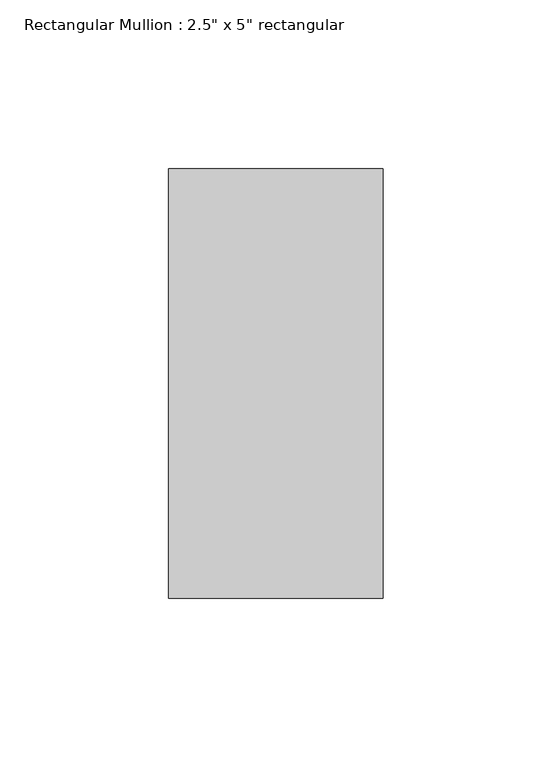
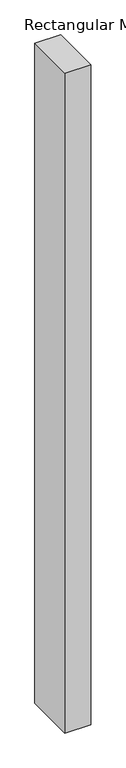
"""IFC4 building model written with IfcOpenShell, lengths in millimetres: member geometry."""

from ifc_helpers import new_model, si_unit, frame, origin, place, context, project, spatial, polyline, outline, extrude, source, transform, mapped, element, save


def member_2501c824(model_context):
    return source(origin(), model_context, "Body", "SweptSolid", [
        extrude(outline(polyline([(0.0, 63.5), (0.0, -63.5), (-63.5, -63.5), (-63.5, 63.5), (0.0, 63.5)])), frame((0.0, 0.0, -1714.5), z_axis=(0.0, 0.0, 1.0), x_axis=(1.0, 0.0, 0.0)), (0.0, 0.0, 1.0), 1714.5),
    ])


if __name__ == "__main__":
    model = new_model("IFC4")
    model_context = context("Model", 3, world=origin())
    ifc_project = project(units=[si_unit("LENGTHUNIT", "METRE", prefix="MILLI")], contexts=[model_context])
    site = spatial("IfcSite", under=ifc_project)
    building = spatial("IfcBuilding", under=site)
    placement = place(None, origin())
    member_shape = member_2501c824(model_context)
    element("IfcMember", 1, ObjectType="Rectangular Mullion : 2.5\" x 5\" rectangular", at=placement, inside=building, context=model_context, shape_type="MappedRepresentation", body=[
        mapped(member_shape, transform((0.0, 0.0, 0.0), x_axis=(1.0, 0.0, 0.0), y_axis=(0.0, 1.0, 0.0), z_axis=(0.0, 0.0, 1.0))),
    ])
    save(model, "model.ifc")

# Revit data of these elements
# Type "Rectangular Mullion : 2.5\" x 5\" rectangular"
#   built-in parameter 1007304 = 0.416667 (stored number, unit not read)
#   built-in parameter 1007301 = 0.104167 (stored number, unit not read)
#   built-in parameter 1007300 = 0.104167 (stored number, unit not read)
# Element 1 (IfcMember, "Rectangular Mullion : 2.5\" x 5\" rectangular")
#   Materials on its faces: "Aluminum"
# Materials
#   "Aluminum": class "Metal", colour RGB 247 247 247, transparency 0, Description = "Aluminum 6061", Cost = 0
